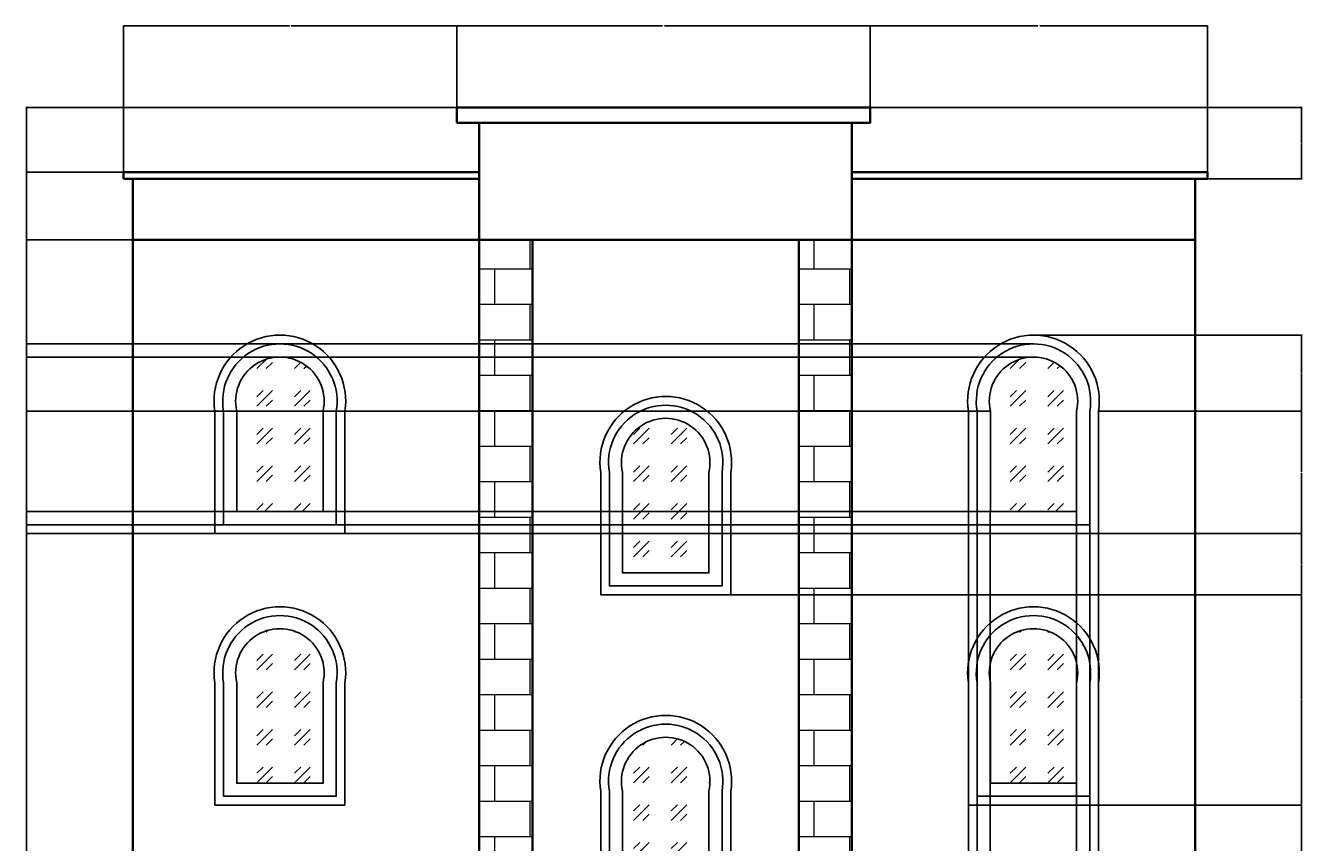
# Model space of a CAD drawing. Units: inches. Extents: x -19 to 556, y -28 to 766.
# Tile 3 of 3: x -19 to 556, y 397 to 766. Entities that reach past the tile are written whole.
import ezdxf

# ---------------------------------------------------------------- set-up
doc = ezdxf.new("R2010")
doc.units = ezdxf.units.IN
doc.header["$MEASUREMENT"] = 0
for name, color, linetype, lineweight in [('A-ANNO-DIMS', 2, 'Continuous', 18), ('A-ELEV', 7, 'Continuous', 35), ('A-GLAZ', 4, 'Continuous', 25), ('A-GLAZ-PATT', 252, 'Continuous', 13), ('A-ROOF', 7, 'Continuous', 35), ('A-WALL-PATT', 8, 'Continuous', 13)]:
    doc.layers.add(name, color=color, linetype=linetype, lineweight=lineweight)
doc.styles.get("Standard").update_dxf_attribs({"font": 'arial.ttf'})
doc.dimstyles.get("Standard").update_dxf_attribs({"dimtxt": 0.18, "dimasz": 0.18, "dimexe": 0.18, "dimexo": 0.0625, "dimgap": 0.09, "dimtad": 0, "dimtih": 1, "dimtoh": 1, "dimdec": 4, "dimzin": 0, "dimdsep": 46, "dimtxsty": 'Standard', "dimcen": 0.09, "dimadec": 0, "dimazin": 0, "dimtfac": 1, "dimtdec": 4, "dimtofl": 0, "dimtmove": 0, "dimatfit": 3, "dimfxl": 1, "dimtolj": 1, "dimtzin": 0, "dimarcsym": 0})

# ---------------------------------------------------------------- blocks, each defined once
blk = doc.blocks.new('WIN-ARCHED')
for points in [[(65.94, 237.64), (65.94, 182.48), (124.55, 182.48), (124.55, 237.64, 1.168317)], [(69.88, 237.64), (69.88, 186.43), (120.6, 186.43), (120.6, 237.64, 1.194508)], [(75.8, 237.64), (75.8, 192.35), (114.68, 192.35), (114.68, 237.64, 1.253731)]]:
    blk.add_lwpolyline(points, format="xyb", close=True)
blk = doc.blocks.new('*D8')
at = {"layer": 'A-ANNO-DIMS', "color": 0, "lineweight": -2, "transparency": 16777216}
for p, q in [((24.79, 699.52), (24.79, 765.64)), ((24.97, 765.46), (99.5, 765.46)), ((174.8, 765.46), (100.27, 765.46)), ((174.98, 721.77), (174.98, 765.64))]:
    blk.add_line(p, q, dxfattribs=at)
at = {"layer": 'A-ANNO-DIMS', "color": 0, "transparency": 16777216}
for points in [[(24.97, 765.49), (24.97, 765.43), (24.79, 765.46)], [(174.8, 765.49), (174.8, 765.43), (174.98, 765.46)]]:
    blk.add_solid(points, dxfattribs=at)
at = {"layer": 'Defpoints', "color": 0, "transparency": 16777216}
for p in [(174.98, 765.46), (174.98, 721.71), (24.79, 699.46)]:
    blk.add_point(p, dxfattribs=at)
at = {"layer": 'A-ANNO-DIMS', "color": 0, "transparency": 16777216, "insert": (99.88, 765.46), "char_height": 0.18, "attachment_point": 5}
blk.add_mtext('\\A1;150.2', dxfattribs=at)
blk = doc.blocks.new('*D9')
at = {"layer": 'A-ANNO-DIMS', "color": 0, "lineweight": -2, "transparency": 16777216}
for p, q in [((174.98, 721.77), (174.98, 765.64)), ((175.16, 765.46), (267.6, 765.46)), ((360.96, 765.46), (268.51, 765.46)), ((361.14, 721.77), (361.14, 765.64))]:
    blk.add_line(p, q, dxfattribs=at)
at = {"layer": 'A-ANNO-DIMS', "color": 0, "transparency": 16777216}
for points in [[(175.16, 765.49), (175.16, 765.43), (174.98, 765.46)], [(360.96, 765.49), (360.96, 765.43), (361.14, 765.46)]]:
    blk.add_solid(points, dxfattribs=at)
at = {"layer": 'Defpoints', "color": 0, "transparency": 16777216}
for p in [(361.14, 765.46), (174.98, 721.71), (361.14, 721.71)]:
    blk.add_point(p, dxfattribs=at)
at = {"layer": 'A-ANNO-DIMS', "color": 0, "transparency": 16777216, "insert": (268.06, 765.46), "char_height": 0.18, "attachment_point": 5}
blk.add_mtext('\\A1;186.16', dxfattribs=at)
blk = doc.blocks.new('*D10')
at = {"layer": 'A-ANNO-DIMS', "color": 0, "lineweight": -2, "transparency": 16777216}
for p, q in [((361.14, 721.77), (361.14, 765.64)), ((361.32, 765.46), (436.7, 765.46)), ((513, 765.46), (437.61, 765.46)), ((513.18, 699.52), (513.18, 765.64))]:
    blk.add_line(p, q, dxfattribs=at)
at = {"layer": 'A-ANNO-DIMS', "color": 0, "transparency": 16777216}
for points in [[(361.32, 765.49), (361.32, 765.43), (361.14, 765.46)], [(513, 765.49), (513, 765.43), (513.18, 765.46)]]:
    blk.add_solid(points, dxfattribs=at)
at = {"layer": 'Defpoints', "color": 0, "transparency": 16777216}
for p in [(513.18, 765.46), (361.14, 721.71), (513.18, 699.46)]:
    blk.add_point(p, dxfattribs=at)
at = {"layer": 'A-ANNO-DIMS', "color": 0, "transparency": 16777216, "insert": (437.16, 765.46), "char_height": 0.18, "attachment_point": 5}
blk.add_mtext('\\A1;152.05', dxfattribs=at)
blk = doc.blocks.new('*D11')
at = {"layer": 'A-ANNO-DIMS', "color": 0, "lineweight": -2, "transparency": 16777216}
for p, q in [((174.92, 728.71), (-19.15, 728.71)), ((-18.97, 728.53), (-18.97, 369.07)), ((-18.97, 9.25), (-18.97, 368.71)), ((28.92, 9.07), (-19.15, 9.07))]:
    blk.add_line(p, q, dxfattribs=at)
at = {"layer": 'A-ANNO-DIMS', "color": 0, "transparency": 16777216}
for points in [[(-19, 728.53), (-18.94, 728.53), (-18.97, 728.71)], [(-19, 9.25), (-18.94, 9.25), (-18.97, 9.07)]]:
    blk.add_solid(points, dxfattribs=at)
at = {"layer": 'Defpoints', "color": 0, "transparency": 16777216}
for p in [(-18.97, 728.71), (174.98, 728.71), (28.98, 9.07)]:
    blk.add_point(p, dxfattribs=at)
at = {"layer": 'A-ANNO-DIMS', "color": 0, "transparency": 16777216, "insert": (-18.97, 368.89), "char_height": 0.18, "attachment_point": 5}
blk.add_mtext('\\A1;719.6', dxfattribs=at)
blk = doc.blocks.new('*D14')
at = {"layer": 'A-ANNO-DIMS', "color": 0, "lineweight": -2, "transparency": 16777216}
for p, q in [((28.92, 669.07), (-19.15, 669.07)), ((-18.97, 668.89), (-18.97, 413.85)), ((-18.97, 158.44), (-18.97, 413.49)), ((28.92, 158.26), (-19.15, 158.26))]:
    blk.add_line(p, q, dxfattribs=at)
at = {"layer": 'A-ANNO-DIMS', "color": 0, "transparency": 16777216}
for points in [[(-19, 668.89), (-18.94, 668.89), (-18.97, 669.07)], [(-19, 158.44), (-18.94, 158.44), (-18.97, 158.26)]]:
    blk.add_solid(points, dxfattribs=at)
at = {"layer": 'Defpoints', "color": 0, "transparency": 16777216}
for p in [(-18.97, 669.07), (28.98, 669.07), (28.98, 158.26)]:
    blk.add_point(p, dxfattribs=at)
at = {"layer": 'A-ANNO-DIMS', "color": 0, "transparency": 16777216, "insert": (-18.97, 413.67), "char_height": 0.18, "attachment_point": 5}
blk.add_mtext('\\A1;510.8', dxfattribs=at)
blk = doc.blocks.new('*D15')
at = {"layer": 'A-ANNO-DIMS', "color": 0, "lineweight": -2, "transparency": 16777216}
for p, q in [((24.72, 699.46), (-19.15, 699.46)), ((-18.97, 699.28), (-18.97, 684.45)), ((-18.97, 669.25), (-18.97, 684.09)), ((28.92, 669.07), (-19.15, 669.07))]:
    blk.add_line(p, q, dxfattribs=at)
at = {"layer": 'A-ANNO-DIMS', "color": 0, "transparency": 16777216}
for points in [[(-19, 699.28), (-18.94, 699.28), (-18.97, 699.46)], [(-19, 669.25), (-18.94, 669.25), (-18.97, 669.07)]]:
    blk.add_solid(points, dxfattribs=at)
at = {"layer": 'Defpoints', "color": 0, "transparency": 16777216}
for p in [(-18.97, 699.46), (24.79, 699.46), (28.98, 669.07)]:
    blk.add_point(p, dxfattribs=at)
at = {"layer": 'A-ANNO-DIMS', "color": 0, "transparency": 16777216, "insert": (-18.97, 684.27), "char_height": 0.18, "attachment_point": 5}
blk.add_mtext('\\A1;30.39', dxfattribs=at)
blk = doc.blocks.new('*D16')
at = {"layer": 'A-ANNO-DIMS', "color": 0, "lineweight": -2, "transparency": 16777216}
for p, q in [((361.2, 728.71), (555.75, 728.71)), ((555.57, 728.53), (555.57, 712.78)), ((555.57, 696.66), (555.57, 712.41)), ((507.65, 696.48), (555.75, 696.48))]:
    blk.add_line(p, q, dxfattribs=at)
at = {"layer": 'A-ANNO-DIMS', "color": 0, "transparency": 16777216}
for points in [[(555.54, 728.53), (555.6, 728.53), (555.57, 728.71)], [(555.54, 696.66), (555.6, 696.66), (555.57, 696.48)]]:
    blk.add_solid(points, dxfattribs=at)
at = {"layer": 'Defpoints', "color": 0, "transparency": 16777216}
for p in [(361.14, 728.71), (555.57, 728.71), (507.59, 696.48)]:
    blk.add_point(p, dxfattribs=at)
at = {"layer": 'A-ANNO-DIMS', "color": 0, "transparency": 16777216, "insert": (555.57, 712.59), "char_height": 0.18, "attachment_point": 5}
blk.add_mtext('\\A1;32.23', dxfattribs=at)
blk = doc.blocks.new('*D26')
at = {"layer": 'A-ANNO-DIMS', "color": 0, "lineweight": -2, "transparency": 16777216}
for p, q in [((464.13, 414.2), (555.75, 414.2)), ((555.57, 414.02), (555.57, 389.91)), ((555.57, 365.43), (555.57, 389.55)), ((298.45, 365.25), (555.75, 365.25))]:
    blk.add_line(p, q, dxfattribs=at)
at = {"layer": 'A-ANNO-DIMS', "color": 0, "transparency": 16777216}
for points in [[(555.54, 414.02), (555.6, 414.02), (555.57, 414.2)], [(555.54, 365.43), (555.6, 365.43), (555.57, 365.25)]]:
    blk.add_solid(points, dxfattribs=at)
at = {"layer": 'Defpoints', "color": 0, "transparency": 16777216}
for p in [(464.07, 414.2), (555.57, 414.2), (298.39, 365.25)]:
    blk.add_point(p, dxfattribs=at)
at = {"layer": 'A-ANNO-DIMS', "color": 0, "transparency": 16777216, "insert": (555.57, 389.73), "char_height": 0.18, "attachment_point": 5}
blk.add_mtext('\\A1;48.95', dxfattribs=at)
blk = doc.blocks.new('*D27')
at = {"layer": 'A-ANNO-DIMS', "color": 0, "lineweight": -2, "transparency": 16777216}
for p, q in [((298.45, 509.03), (555.75, 509.03)), ((555.57, 508.85), (555.57, 461.8)), ((555.57, 414.38), (555.57, 461.43)), ((464.13, 414.2), (555.75, 414.2))]:
    blk.add_line(p, q, dxfattribs=at)
at = {"layer": 'A-ANNO-DIMS', "color": 0, "transparency": 16777216}
for points in [[(555.54, 508.85), (555.6, 508.85), (555.57, 509.03)], [(555.54, 414.38), (555.6, 414.38), (555.57, 414.2)]]:
    blk.add_solid(points, dxfattribs=at)
at = {"layer": 'Defpoints', "color": 0, "transparency": 16777216}
for p in [(298.39, 509.03), (555.57, 509.03), (464.07, 414.2)]:
    blk.add_point(p, dxfattribs=at)
at = {"layer": 'A-ANNO-DIMS', "color": 0, "transparency": 16777216, "insert": (555.57, 461.61), "char_height": 0.18, "attachment_point": 5}
blk.add_mtext('\\A1;94.82', dxfattribs=at)
blk = doc.blocks.new('*D28')
at = {"layer": 'A-ANNO-DIMS', "color": 0, "lineweight": -2, "transparency": 16777216}
for p, q in [((464.13, 536.66), (555.75, 536.66)), ((555.57, 536.48), (555.57, 523.02)), ((555.57, 509.21), (555.57, 522.66)), ((298.45, 509.03), (555.75, 509.03))]:
    blk.add_line(p, q, dxfattribs=at)
at = {"layer": 'A-ANNO-DIMS', "color": 0, "transparency": 16777216}
for points in [[(555.54, 536.48), (555.6, 536.48), (555.57, 536.66)], [(555.54, 509.21), (555.6, 509.21), (555.57, 509.03)]]:
    blk.add_solid(points, dxfattribs=at)
at = {"layer": 'Defpoints', "color": 0, "transparency": 16777216}
for p in [(464.07, 536.66), (555.57, 536.66), (298.39, 509.03)]:
    blk.add_point(p, dxfattribs=at)
at = {"layer": 'A-ANNO-DIMS', "color": 0, "transparency": 16777216, "insert": (555.57, 522.84), "char_height": 0.18, "attachment_point": 5}
blk.add_mtext('\\A1;27.633', dxfattribs=at)
blk = doc.blocks.new('*D42')
at = {"layer": 'A-ANNO-DIMS', "color": 0, "lineweight": -2, "transparency": 16777216}
for p, q in [((405.46, 536.6), (405.46, -27.86)), ((409.4, 540.54), (409.4, -27.86)), ((405.64, -27.68), (407.04, -27.68)), ((409.22, -27.68), (407.82, -27.68))]:
    blk.add_line(p, q, dxfattribs=at)
at = {"layer": 'A-ANNO-DIMS', "color": 0, "transparency": 16777216}
for points in [[(405.64, -27.65), (405.64, -27.71), (405.46, -27.68)], [(409.22, -27.65), (409.22, -27.71), (409.4, -27.68)]]:
    blk.add_solid(points, dxfattribs=at)
at = {"layer": 'Defpoints', "color": 0, "transparency": 16777216}
for p in [(405.46, 536.66), (409.4, 540.61), (409.4, -27.68)]:
    blk.add_point(p, dxfattribs=at)
at = {"layer": 'A-ANNO-DIMS', "color": 0, "transparency": 16777216, "insert": (407.43, -27.68), "char_height": 0.18, "attachment_point": 5}
blk.add_mtext('\\A1;3.946', dxfattribs=at)
blk = doc.blocks.new('*D43')
at = {"layer": 'A-ANNO-DIMS', "color": 0, "lineweight": -2, "transparency": 16777216}
for p, q in [((415.32, 546.46), (415.32, -27.86)), ((409.4, 540.54), (409.4, -27.86)), ((409.58, -27.68), (411.97, -27.68)), ((415.14, -27.68), (412.76, -27.68))]:
    blk.add_line(p, q, dxfattribs=at)
at = {"layer": 'A-ANNO-DIMS', "color": 0, "transparency": 16777216}
for points in [[(409.58, -27.65), (409.58, -27.71), (409.4, -27.68)], [(415.14, -27.65), (415.14, -27.71), (415.32, -27.68)]]:
    blk.add_solid(points, dxfattribs=at)
at = {"layer": 'Defpoints', "color": 0, "transparency": 16777216}
for p in [(415.32, 546.52), (409.4, 540.61), (415.32, -27.68)]:
    blk.add_point(p, dxfattribs=at)
at = {"layer": 'A-ANNO-DIMS', "color": 0, "transparency": 16777216, "insert": (412.36, -27.68), "char_height": 0.18, "attachment_point": 5}
blk.add_mtext('\\A1;5.919', dxfattribs=at)
blk = doc.blocks.new('*D44')
at = {"layer": 'A-ANNO-DIMS', "color": 0, "lineweight": -2, "transparency": 16777216}
for p, q in [((415.32, 546.46), (415.32, -27.86)), ((454.21, 546.46), (454.21, -27.86)), ((415.5, -27.68), (434.37, -27.68)), ((454.03, -27.68), (435.16, -27.68))]:
    blk.add_line(p, q, dxfattribs=at)
at = {"layer": 'A-ANNO-DIMS', "color": 0, "transparency": 16777216}
for points in [[(415.5, -27.65), (415.5, -27.71), (415.32, -27.68)], [(454.03, -27.65), (454.03, -27.71), (454.21, -27.68)]]:
    blk.add_solid(points, dxfattribs=at)
at = {"layer": 'Defpoints', "color": 0, "transparency": 16777216}
for p in [(415.32, 546.52), (454.21, 546.52), (454.21, -27.68)]:
    blk.add_point(p, dxfattribs=at)
at = {"layer": 'A-ANNO-DIMS', "color": 0, "transparency": 16777216, "insert": (434.76, -27.68), "char_height": 0.18, "attachment_point": 5}
blk.add_mtext('\\A1;38.88', dxfattribs=at)
blk = doc.blocks.new('*D45')
at = {"layer": 'A-ANNO-DIMS', "color": 0, "lineweight": -2, "transparency": 16777216}
for p, q in [((454.21, 546.46), (454.21, -27.86)), ((460.12, 540.54), (460.12, -27.86)), ((454.39, -27.68), (456.77, -27.68)), ((459.94, -27.68), (457.56, -27.68))]:
    blk.add_line(p, q, dxfattribs=at)
at = {"layer": 'A-ANNO-DIMS', "color": 0, "transparency": 16777216}
for points in [[(454.39, -27.65), (454.39, -27.71), (454.21, -27.68)], [(459.94, -27.65), (459.94, -27.71), (460.12, -27.68)]]:
    blk.add_solid(points, dxfattribs=at)
at = {"layer": 'Defpoints', "color": 0, "transparency": 16777216}
for p in [(454.21, 546.52), (460.12, 540.61), (460.12, -27.68)]:
    blk.add_point(p, dxfattribs=at)
at = {"layer": 'A-ANNO-DIMS', "color": 0, "transparency": 16777216, "insert": (457.16, -27.68), "char_height": 0.18, "attachment_point": 5}
blk.add_mtext('\\A1;5.919', dxfattribs=at)
blk = doc.blocks.new('*D46')
at = {"layer": 'A-ANNO-DIMS', "color": 0, "lineweight": -2, "transparency": 16777216}
for p, q in [((460.12, 540.54), (460.12, -27.86)), ((464.07, 536.6), (464.07, -27.86)), ((460.3, -27.68), (461.7, -27.68)), ((463.89, -27.68), (462.49, -27.68))]:
    blk.add_line(p, q, dxfattribs=at)
at = {"layer": 'A-ANNO-DIMS', "color": 0, "transparency": 16777216}
for points in [[(460.3, -27.65), (460.3, -27.71), (460.12, -27.68)], [(463.89, -27.65), (463.89, -27.71), (464.07, -27.68)]]:
    blk.add_solid(points, dxfattribs=at)
at = {"layer": 'Defpoints', "color": 0, "transparency": 16777216}
for p in [(460.12, 540.61), (464.07, 536.66), (464.07, -27.68)]:
    blk.add_point(p, dxfattribs=at)
at = {"layer": 'A-ANNO-DIMS', "color": 0, "transparency": 16777216, "insert": (462.1, -27.68), "char_height": 0.18, "attachment_point": 5}
blk.add_mtext('\\A1;3.946', dxfattribs=at)
blk = doc.blocks.new('*D47')
at = {"layer": 'A-ANNO-DIMS', "color": 0, "lineweight": -2, "transparency": 16777216}
for p, q in [((409.34, 540.61), (-19.15, 540.61)), ((405.39, 536.66), (-19.15, 536.66)), ((-18.97, 540.43), (-18.97, 538.81)), ((-18.97, 536.84), (-18.97, 538.45))]:
    blk.add_line(p, q, dxfattribs=at)
at = {"layer": 'A-ANNO-DIMS', "color": 0, "transparency": 16777216}
for points in [[(-19, 540.43), (-18.94, 540.43), (-18.97, 540.61)], [(-19, 536.84), (-18.94, 536.84), (-18.97, 536.66)]]:
    blk.add_solid(points, dxfattribs=at)
at = {"layer": 'Defpoints', "color": 0, "transparency": 16777216}
for p in [(-18.97, 540.61), (405.46, 536.66), (409.4, 540.61)]:
    blk.add_point(p, dxfattribs=at)
at = {"layer": 'A-ANNO-DIMS', "color": 0, "transparency": 16777216, "insert": (-18.97, 538.63), "char_height": 0.18, "attachment_point": 5}
blk.add_mtext('\\A1;3.946', dxfattribs=at)
blk = doc.blocks.new('*D48')
at = {"layer": 'A-ANNO-DIMS', "color": 0, "lineweight": -2, "transparency": 16777216}
for p, q in [((415.26, 546.52), (-19.15, 546.52)), ((-18.97, 546.34), (-18.97, 543.75)), ((-18.97, 540.79), (-18.97, 543.38)), ((409.34, 540.61), (-19.15, 540.61))]:
    blk.add_line(p, q, dxfattribs=at)
at = {"layer": 'A-ANNO-DIMS', "color": 0, "transparency": 16777216}
for points in [[(-19, 546.34), (-18.94, 546.34), (-18.97, 546.52)], [(-19, 540.79), (-18.94, 540.79), (-18.97, 540.61)]]:
    blk.add_solid(points, dxfattribs=at)
at = {"layer": 'Defpoints', "color": 0, "transparency": 16777216}
for p in [(-18.97, 546.52), (415.32, 546.52), (409.4, 540.61)]:
    blk.add_point(p, dxfattribs=at)
at = {"layer": 'A-ANNO-DIMS', "color": 0, "transparency": 16777216, "insert": (-18.97, 543.57), "char_height": 0.18, "attachment_point": 5}
blk.add_mtext('\\A1;5.919', dxfattribs=at)
blk = doc.blocks.new('*D49')
at = {"layer": 'A-ANNO-DIMS', "color": 0, "lineweight": -2, "transparency": 16777216}
for p, q in [((415.26, 591.81), (-19.15, 591.81)), ((-18.97, 591.63), (-18.97, 569.35)), ((-18.97, 546.7), (-18.97, 568.99)), ((415.26, 546.52), (-19.15, 546.52))]:
    blk.add_line(p, q, dxfattribs=at)
at = {"layer": 'A-ANNO-DIMS', "color": 0, "transparency": 16777216}
for points in [[(-19, 591.63), (-18.94, 591.63), (-18.97, 591.81)], [(-19, 546.7), (-18.94, 546.7), (-18.97, 546.52)]]:
    blk.add_solid(points, dxfattribs=at)
at = {"layer": 'Defpoints', "color": 0, "transparency": 16777216}
for p in [(-18.97, 591.81), (415.32, 591.81), (415.32, 546.52)]:
    blk.add_point(p, dxfattribs=at)
at = {"layer": 'A-ANNO-DIMS', "color": 0, "transparency": 16777216, "insert": (-18.97, 569.17), "char_height": 0.18, "attachment_point": 5}
blk.add_mtext('\\A1;45.29', dxfattribs=at)
blk = doc.blocks.new('*D50')
at = {"layer": 'A-ANNO-DIMS', "color": 0, "lineweight": -2, "transparency": 16777216}
for p, q in [((434.7, 616.19), (-19.15, 616.19)), ((-18.97, 616.01), (-18.97, 604.18)), ((-18.97, 591.99), (-18.97, 603.82)), ((415.26, 591.81), (-19.15, 591.81))]:
    blk.add_line(p, q, dxfattribs=at)
at = {"layer": 'A-ANNO-DIMS', "color": 0, "transparency": 16777216}
for points in [[(-19, 616.01), (-18.94, 616.01), (-18.97, 616.19)], [(-19, 591.99), (-18.94, 591.99), (-18.97, 591.81)]]:
    blk.add_solid(points, dxfattribs=at)
at = {"layer": 'Defpoints', "color": 0, "transparency": 16777216}
for p in [(-18.97, 616.19), (434.76, 616.19), (415.32, 591.81)]:
    blk.add_point(p, dxfattribs=at)
at = {"layer": 'A-ANNO-DIMS', "color": 0, "transparency": 16777216, "insert": (-18.97, 604), "char_height": 0.18, "attachment_point": 5}
blk.add_mtext('\\A1;24.374', dxfattribs=at)
blk = doc.blocks.new('*D51')
at = {"layer": 'A-ANNO-DIMS', "color": 0, "lineweight": -2, "transparency": 16777216}
for p, q in [((464.13, 591.81), (555.75, 591.81)), ((555.57, 591.63), (555.57, 564.42)), ((555.57, 536.84), (555.57, 564.05)), ((464.13, 536.66), (555.75, 536.66))]:
    blk.add_line(p, q, dxfattribs=at)
at = {"layer": 'A-ANNO-DIMS', "color": 0, "transparency": 16777216}
for points in [[(555.54, 591.63), (555.6, 591.63), (555.57, 591.81)], [(555.54, 536.84), (555.6, 536.84), (555.57, 536.66)]]:
    blk.add_solid(points, dxfattribs=at)
at = {"layer": 'Defpoints', "color": 0, "transparency": 16777216}
for p in [(464.07, 591.81), (555.57, 591.81), (464.07, 536.66)]:
    blk.add_point(p, dxfattribs=at)
at = {"layer": 'A-ANNO-DIMS', "color": 0, "transparency": 16777216, "insert": (555.57, 564.24), "char_height": 0.18, "attachment_point": 5}
blk.add_mtext('\\A1;55.15', dxfattribs=at)
blk = doc.blocks.new('*D52')
at = {"layer": 'A-ANNO-DIMS', "color": 0, "lineweight": -2, "transparency": 16777216}
for p, q in [((434.83, 626.05), (555.75, 626.05)), ((555.57, 625.87), (555.57, 609.11)), ((555.57, 591.99), (555.57, 608.75)), ((464.13, 591.81), (555.75, 591.81))]:
    blk.add_line(p, q, dxfattribs=at)
at = {"layer": 'A-ANNO-DIMS', "color": 0, "transparency": 16777216}
for points in [[(555.54, 625.87), (555.6, 625.87), (555.57, 626.05)], [(555.54, 591.99), (555.6, 591.99), (555.57, 591.81)]]:
    blk.add_solid(points, dxfattribs=at)
at = {"layer": 'Defpoints', "color": 0, "transparency": 16777216}
for p in [(434.76, 626.05), (555.57, 626.05), (464.07, 591.81)]:
    blk.add_point(p, dxfattribs=at)
at = {"layer": 'A-ANNO-DIMS', "color": 0, "transparency": 16777216, "insert": (555.57, 608.93), "char_height": 0.18, "attachment_point": 5}
blk.add_mtext('\\A1;34.24', dxfattribs=at)
blk = doc.blocks.new('*D53')
at = {"layer": 'A-ANNO-DIMS', "color": 0, "lineweight": -2, "transparency": 16777216}
for p, q in [((434.7, 622.11), (-19.15, 622.11)), ((-18.97, 621.93), (-18.97, 607.14)), ((-18.97, 591.99), (-18.97, 606.78)), ((409.34, 591.81), (-19.15, 591.81))]:
    blk.add_line(p, q, dxfattribs=at)
at = {"layer": 'A-ANNO-DIMS', "color": 0, "transparency": 16777216}
for points in [[(-19, 621.93), (-18.94, 621.93), (-18.97, 622.11)], [(-19, 591.99), (-18.94, 591.99), (-18.97, 591.81)]]:
    blk.add_solid(points, dxfattribs=at)
at = {"layer": 'Defpoints', "color": 0, "transparency": 16777216}
for p in [(-18.97, 622.11), (434.76, 622.11), (409.4, 591.81)]:
    blk.add_point(p, dxfattribs=at)
at = {"layer": 'A-ANNO-DIMS', "color": 0, "transparency": 16777216, "insert": (-18.97, 606.96), "char_height": 0.18, "attachment_point": 5}
blk.add_mtext('\\A1;30.293', dxfattribs=at)

msp = doc.modelspace()

# ---------------------------------------------------------------- hatches: boundary and pattern name
at = {"layer": 'A-GLAZ-PATT'}
h = msp.add_hatch(dxfattribs=at)
h.set_pattern_fill('GOST_GLASS', color=256, scale=2)
h.set_pattern_definition([(45, (0, 0), (16.97056, 0), [10, -14]), (45, (4.243, 0), (16.97056, 0), [4, -20]), (45, (0, 4.243), (16.97056, 0), [4, -20])])
h.paths.add_polyline_path([(114.6834, 591.8123, 1.25373075), (75.801, 591.8123), (75.801, 546.5249), (114.6834, 546.5249)])
h.paths.add_polyline_path([(454.2051, 591.8123, 1.25373075), (415.3227, 591.8123), (415.3227, 546.5249), (454.2051, 546.5249)])
h.paths.add_polyline_path([(288.5244, 564.1792, 1.25373075), (249.6421, 564.1792), (249.6421, 518.8919), (288.5244, 518.8919)])
h.paths.add_polyline_path([(114.6834, 469.356, 1.25373075), (75.801, 469.356), (75.801, 424.0687), (114.6834, 424.0687)])
h.paths.add_polyline_path([(288.5244, 420.4043, 1.25373075), (249.6421, 420.4043), (249.6421, 375.1169), (288.5244, 375.1169)])
h.paths.add_polyline_path([(454.2051, 469.356, 1.25373075), (415.3227, 469.356), (415.3227, 424.0687), (454.2051, 424.0687)])
h.paths.add_polyline_path([(454.2051, 353.5792, 1.25373075), (415.3227, 353.5792), (415.3227, 308.2919), (454.2051, 308.2919)])
h.paths.add_polyline_path([(454.2051, 237.6357, 1.25373075), (415.3227, 237.6357), (415.3227, 192.3483), (454.2051, 192.3483)])
h.paths.add_polyline_path([(288.5244, 280.5161, 1.25373075), (249.6421, 280.5161), (249.6421, 235.2288), (288.5244, 235.2288)])
h.paths.add_polyline_path([(114.6834, 237.6357, 1.25373075), (75.801, 237.6357), (75.801, 192.3483), (114.6834, 192.3483)])
h.paths.add_polyline_path([(114.6834, 353.5792, 1.25373075), (75.801, 353.5792), (75.801, 308.2919), (114.6834, 308.2919)])
at = {"layer": 'A-WALL-PATT'}
h = msp.add_hatch(dxfattribs=at)
h.set_pattern_fill('AR-B816', color=256, scale=2)
h.paths.add_polyline_path([(208.9833, 669.0741), (184.9833, 669.0741), (184.9833, 129.0741), (184.9833, 9.0741), (208.9833, 9.0741), (208.9833, 129.0741)])
h.paths.add_polyline_path([(352.9833, 669.0741), (328.9833, 669.0741), (328.9833, 129.0741), (328.9833, 9.0741), (352.9833, 9.0741), (352.9833, 129.0741)])

# ---------------------------------------------------------------- linework, layer by layer
at = {"layer": 'A-ELEV'}
for p, q in [((184.9833, 669.0741), (184.9833, 129.0741)), ((328.9833, 129.0741), (328.9833, 669.0741)), ((352.9833, 669.0741), (352.9833, 129.0741))]:
    msp.add_line(p, q, dxfattribs=at)
for points in [[(507.6136, 158.26), (507.6136, 669.0741), (28.9833, 669.0741), (28.9833, 158.26)], [(208.9833, 669.0741), (208.9833, 129.0741), (208.9833, 9.0741)]]:
    msp.add_lwpolyline(points, dxfattribs=at)
at = {"layer": 'A-ROOF'}
for points in [[(174.98, 721.7111), (361.1359, 721.7111), (361.1359, 728.7105), (174.98, 728.7105)], [(184.9833, 669.0741), (352.9833, 669.0741), (352.9833, 721.7111), (184.9833, 721.7111)], [(24.7851, 696.4776), (184.9833, 696.4776), (184.9833, 699.4612), (24.7851, 699.4612)], [(28.9833, 669.0741), (184.9833, 669.0741), (184.9833, 696.4776), (28.9833, 696.4776)], [(352.9833, 696.4776), (513.1815, 696.4776), (513.1815, 699.4612), (352.9833, 699.4612)], [(352.9833, 669.0741), (507.5909, 669.0741), (507.5909, 696.4776), (352.9833, 696.4776)]]:
    msp.add_lwpolyline(points, close=True, dxfattribs=at)

# ---------------------------------------------------------------- block references
at = {"layer": 'A-GLAZ'}
for p in [(0, 354.1766), (339.5217, 354.1766), (173.841, 326.5436), (0, 231.7204), (339.5217, 231.7204), (173.841, 182.7686)]:
    msp.add_blockref('WIN-ARCHED', p, dxfattribs=at)

# ---------------------------------------------------------------- dimensions: what is measured, and where the dimension line sits
at = {"layer": 'A-ANNO-DIMS'}
for base, p1, p2, override, picture, middle in [((174.98, 765.4605), (24.7851, 699.4612), (174.98, 721.7111), {"dimdec": 1, "dimlfac": 1, "dimrnd": 0, "dimzin": 0, "dimdsep": 46, "dimlunit": 2}, '*D8', (99.8826, 765.4605)), ((361.1359, 765.4605), (174.98, 721.7111), (361.1359, 721.7111), {"dimdec": 2, "dimlfac": 1, "dimrnd": 0, "dimzin": 0, "dimdsep": 46, "dimlunit": 2}, '*D9', (268.058, 765.4605)), ((513.1815, 765.4605), (361.1359, 721.7111), (513.1815, 699.4612), {"dimdec": 2, "dimlfac": 1, "dimrnd": 0, "dimzin": 0, "dimdsep": 46, "dimlunit": 2}, '*D10', (437.1587, 765.4605)), ((415.3227, -27.6759), (409.4034, 540.6055), (415.3227, 546.5249), {"dimdec": 3, "dimlfac": 1, "dimrnd": 0, "dimzin": 0, "dimdsep": 46, "dimlunit": 2}, '*D43', (412.3631, -27.6759)), ((454.2051, -27.6759), (415.3227, 546.5249), (454.2051, 546.5249), {"dimdec": 2, "dimlfac": 1, "dimrnd": 0, "dimzin": 0, "dimdsep": 46, "dimlunit": 2}, '*D44', (434.7639, -27.6759)), ((460.1245, -27.6759), (454.2051, 546.5249), (460.1245, 540.6055), {"dimdec": 3, "dimlfac": 1, "dimrnd": 0, "dimzin": 0, "dimdsep": 46, "dimlunit": 2}, '*D45', (457.1648, -27.6759)), ((409.4034, -27.6759), (405.4571, 536.6593), (409.4034, 540.6055), {"dimdec": 3, "dimlfac": 1, "dimrnd": 0, "dimzin": 0, "dimdsep": 46, "dimlunit": 2}, '*D42', (407.4302, -27.6759)), ((464.0708, -27.6759), (460.1245, 540.6055), (464.0708, 536.6593), {"dimdec": 3, "dimlfac": 1, "dimrnd": 0, "dimzin": 0, "dimdsep": 46, "dimlunit": 2}, '*D46', (462.0976, -27.6759))]:
    dim = msp.add_linear_dim(base=base, p1=p1, p2=p2, dimstyle='Standard', override=override, dxfattribs=at)
    dim.commit()
    dim.dimension.update_dxf_attribs({"geometry": picture, "text_midpoint": middle})
for base, p1, p2, override, picture, middle in [((-18.9726, 728.7105), (28.9833, 9.0741), (174.98, 728.7105), {"dimdec": 1, "dimlfac": 1, "dimrnd": 0, "dimzin": 0, "dimdsep": 46, "dimlunit": 2}, '*D11', (-18.9726, 368.8923)), ((555.5695, 728.7105), (507.5909, 696.4776), (361.1359, 728.7105), {"dimdec": 2, "dimlfac": 1, "dimrnd": 0, "dimzin": 0, "dimdsep": 46, "dimlunit": 2}, '*D16', (555.5695, 712.594)), ((-18.9726, 699.4612), (28.9833, 669.0741), (24.7851, 699.4612), {"dimdec": 2, "dimlfac": 1, "dimrnd": 0, "dimzin": 0, "dimdsep": 46, "dimlunit": 2}, '*D15', (-18.9726, 684.2676)), ((-18.9726, 669.0741), (28.9833, 158.26), (28.9833, 669.0741), {"dimdec": 1, "dimlfac": 1, "dimrnd": 0, "dimzin": 0, "dimdsep": 46, "dimlunit": 2}, '*D14', (-18.9726, 413.6671)), ((-18.9726, 622.1057), (409.4034, 591.8123), (434.7639, 622.1057), {"dimdec": 3, "dimlfac": 1, "dimrnd": 0, "dimzin": 0, "dimdsep": 46, "dimlunit": 2}, '*D53', (-18.9726, 606.959)), ((555.5695, 626.0519), (464.0708, 591.8123), (434.7639, 626.0519), {"dimdec": 2, "dimlfac": 1, "dimrnd": 0, "dimzin": 0, "dimdsep": 46, "dimlunit": 2}, '*D52', (555.5695, 608.9321)), ((-18.9726, 616.1863), (415.3227, 591.8123), (434.7639, 616.1863), {"dimdec": 3, "dimlfac": 1, "dimrnd": 0, "dimzin": 0, "dimdsep": 46, "dimlunit": 2}, '*D50', (-18.9726, 603.9993)), ((-18.9726, 591.8123), (415.3227, 546.5249), (415.3227, 591.8123), {"dimdec": 2, "dimlfac": 1, "dimrnd": 0, "dimzin": 0, "dimdsep": 46, "dimlunit": 2}, '*D49', (-18.9726, 569.1686)), ((555.5695, 591.8123), (464.0708, 536.6593), (464.0708, 591.8123), {"dimdec": 2, "dimlfac": 1, "dimrnd": 0, "dimzin": 0, "dimdsep": 46, "dimlunit": 2}, '*D51', (555.5695, 564.2358)), ((-18.9726, 546.5249), (409.4034, 540.6055), (415.3227, 546.5249), {"dimdec": 3, "dimlfac": 1, "dimrnd": 0, "dimzin": 0, "dimdsep": 46, "dimlunit": 2}, '*D48', (-18.9726, 543.5652)), ((-18.9726, 540.6055), (405.4571, 536.6593), (409.4034, 540.6055), {"dimdec": 3, "dimlfac": 1, "dimrnd": 0, "dimzin": 0, "dimdsep": 46, "dimlunit": 2}, '*D47', (-18.9726, 538.6324)), ((555.5695, 536.6593), (298.3901, 509.0262), (464.0708, 536.6593), {"dimdec": 3, "dimlfac": 1, "dimrnd": 0, "dimzin": 0, "dimdsep": 46, "dimlunit": 2}, '*D28', (555.5695, 522.8428)), ((555.5695, 509.0262), (464.0708, 414.203), (298.3901, 509.0262), {"dimdec": 2, "dimlfac": 1, "dimrnd": 0, "dimzin": 0, "dimdsep": 46, "dimlunit": 2}, '*D27', (555.5695, 461.6146)), ((555.5695, 414.203), (298.3901, 365.2513), (464.0708, 414.203), {"dimdec": 2, "dimlfac": 1, "dimrnd": 0, "dimzin": 0, "dimdsep": 46, "dimlunit": 2}, '*D26', (555.5695, 389.7272))]:
    dim = msp.add_linear_dim(base=base, p1=p1, p2=p2, angle=90, dimstyle='Standard', override=override, dxfattribs=at)
    dim.commit()
    dim.dimension.update_dxf_attribs({"geometry": picture, "text_midpoint": middle})

doc.saveas('drawing.dxf')
